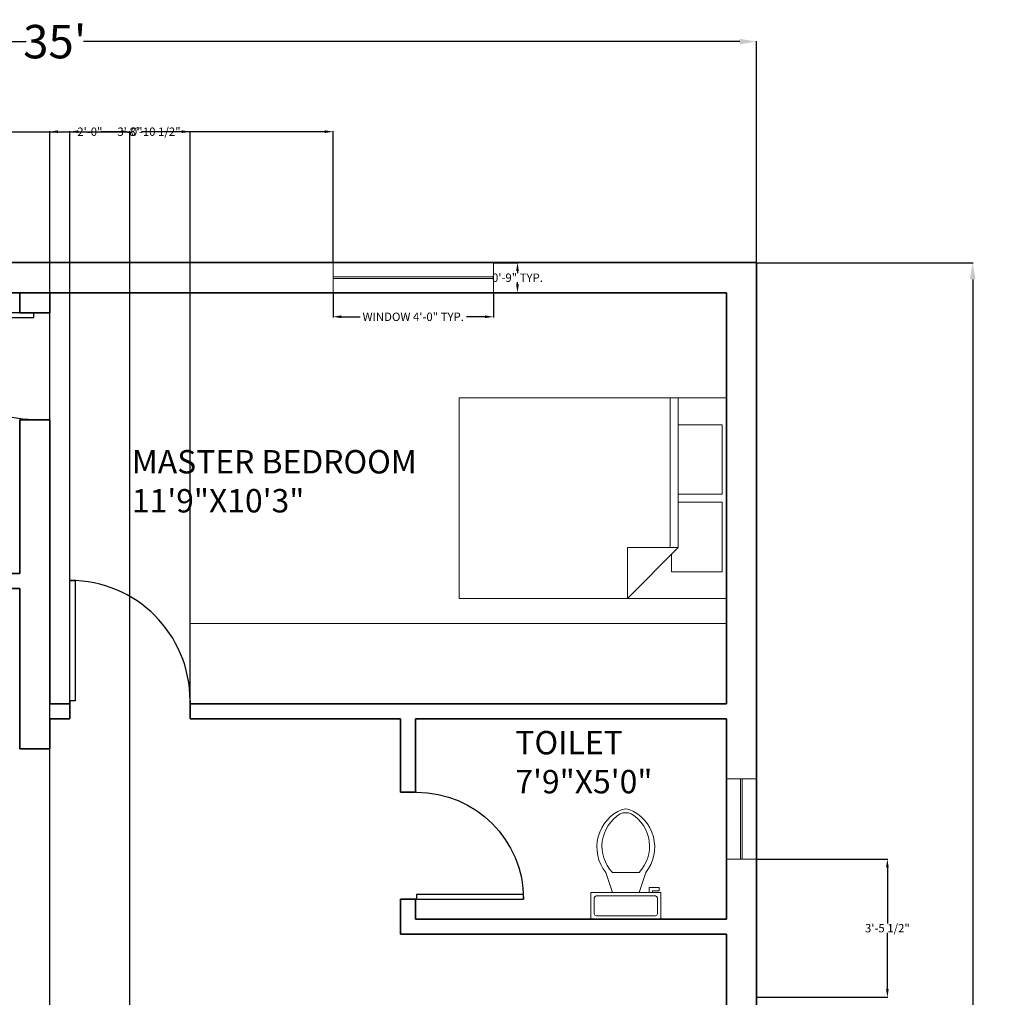
# Model space of a CAD drawing. Units: inches. Extents: x 481 to 2783, y 1975 to 3327.
# Tile 9 of 13: x 1574 to 1869, y 3034 to 3327. Entities that reach past the tile are written whole.
import ezdxf

# ---------------------------------------------------------------- set-up
doc = ezdxf.new("R2010")
doc.units = ezdxf.units.IN
doc.header["$MEASUREMENT"] = 0
for name, color, linetype, lineweight in [('A-ANNO-DIMS', 50, 'Continuous', 18), ('A-AREA-IDEN', 50, 'Continuous', 18), ('A-FLOR-CASE', 61, 'Continuous', 18), ('A-FLOR-FIXT', 61, 'Continuous', 18), ('A-FURN', 61, 'Continuous', 18), ('A-WALL', 40, 'Continuous', 35), ('DOORS', 10, 'Continuous', 25), ('WINDOWS', 220, 'Continuous', 20)]:
    doc.layers.add(name, color=color, linetype=linetype, lineweight=lineweight)
doc.styles.get("Standard").update_dxf_attribs({"font": 'arial.ttf'})
doc.dimstyles.get("Standard").update_dxf_attribs({"dimtxt": 2.5, "dimasz": 2.5, "dimexe": 0.18, "dimexo": 0.0625, "dimgap": 0.09, "dimtad": 0, "dimtih": 1, "dimtoh": 1, "dimzin": 0, "dimdsep": 46, "dimlunit": 3, "dimtxsty": 'Standard', "dimcen": 0.09, "dimadec": 0, "dimazin": 0, "dimtfac": 1, "dimtofl": 0, "dimtmove": 0, "dimatfit": 3, "dimfxl": 1, "dimtolj": 1, "dimtzin": 0, "dimarcsym": 0})

# ---------------------------------------------------------------- blocks, each defined once
blk = doc.blocks.new('*U2')
for p, q in [((0, 0), (0, -6)), ((40, 0), (40, -6))]:
    blk.add_line(p, q)
blk.add_lwpolyline([(0, 0), (0, 40), (1.75, 40), (1.75, 0)], close=True)
blk.add_arc((0, 0), 40, 0, 90)
blk = doc.blocks.new('Bed - Queen')
for p, q in [((0, -80.00003), (0, 0)), ((0, 0), (59.99999, 0)), ((59.99999, 0), (59.99999, -80.00003)), ((7.99999, -1.2), (28.79998, -1.2)), ((7.99999, -14.4), (7.99999, -1.2)), ((28.79998, -1.2), (28.79998, -14.4)), ((31.19999, -1.2), (51.99999, -1.2)), ((31.19999, -14.4), (31.19999, -1.2)), ((51.99999, -1.2), (51.99999, -16.4)), ((0, -14.4), (44.8, -14.4)), ((59.99999, -29.6), (44.8, -14.4)), ((44.8, -14.4), (44.8, -29.6)), ((44.8, -16.8), (0, -16.8)), ((51.99999, -16.4), (46.79936, -16.4)), ((44.8, -29.6), (59.99999, -29.6)), ((59.99999, -80.00003), (0, -80.00003))]:
    blk.add_line(p, q)
blk = doc.blocks.new('Toilet - top')
for p, q in [((9.5, -6), (9.5, -2)), ((-10, -8.5), (-8, -8.5)), ((-10, -9.5), (-10, -8.5)), ((-8, -8.5), (-8, -8)), ((-7, -8), (-7, -9.5)), ((-4, -8), (-6, -14)), ((4, -8), (6, -14)), ((-7, -9.5), (-10, -9.5)), ((4, -14), (-4, -14))]:
    blk.add_line(p, q)
blk.add_lwpolyline([(10.5, -8), (10.5, 0), (-10.5, 0), (-10.5, -8)], close=True)
for points in [[(-9.5, -2), (-9.5, -6)], [(8.5, -1), (-8.5, -1)], [(-8.5, -7), (8.5, -7)]]:
    blk.add_lwpolyline(points)
for centre, radius, start, end in [((-8.62, -1.88), 0.884, 81.8699, 188.1301), ((8.62, -1.88), 0.884, 351.8699, 98.1301), ((-8.62, -6.12), 0.884, 171.8699, 278.1301), ((8.62, -6.12), 0.884, 261.8699, 8.1301), ((3.52, -21.58), 12.17, 141.4691, 247.9714), ((4.2, -21.82), 11.33, 136.3677, 238.9468), ((-3.52, -21.58), 12.17, 292.0284, 38.5307), ((-4.2, -21.82), 11.33, 301.053, 43.6321), ((0, -27.88), 4, 245.7318, 294.2682), ((0, -29), 4, 254.8605, 285.1395)]:
    blk.add_arc(centre, radius, start, end)
blk = doc.blocks.new('*D23')
at = {"layer": 'A-ANNO-DIMS', "color": 0, "lineweight": -2, "transparency": 16777216}
for p, q in [((1794.5, 3254.32), (1859.35, 3254.32)), ((1859.17, 3249.32), (1859.17, 2959.52)), ((1859.17, 2659.32), (1859.17, 2949.13)), ((1794.5, 2654.32), (1859.35, 2654.32))]:
    blk.add_line(p, q, dxfattribs=at)
at = {"layer": 'A-ANNO-DIMS', "color": 0, "transparency": 16777216}
for points in [[(1858.33, 3249.32), (1860, 3249.32), (1859.17, 3254.32)], [(1858.33, 2659.32), (1860, 2659.32), (1859.17, 2654.32)]]:
    blk.add_solid(points, dxfattribs=at)
at = {"layer": 'Defpoints', "color": 0, "transparency": 16777216}
for p in [(1794.44, 3254.32), (1794.44, 2654.32), (1859.17, 2654.32)]:
    blk.add_point(p, dxfattribs=at)
at = {"layer": 'A-ANNO-DIMS', "color": 0, "transparency": 16777216, "insert": (1859.17, 2954.32), "char_height": 10, "attachment_point": 5}
blk.add_mtext("\\A1;50'", dxfattribs=at)
blk = doc.blocks.new('*D24')
at = {"layer": 'A-ANNO-DIMS', "color": 0, "lineweight": -2, "transparency": 16777216}
for p, q in [((1374.44, 3254.39), (1374.44, 3320.66)), ((1379.44, 3320.48), (1575.87, 3320.48)), ((1789.44, 3320.48), (1593.01, 3320.48)), ((1794.44, 3254.39), (1794.44, 3320.66))]:
    blk.add_line(p, q, dxfattribs=at)
at = {"layer": 'A-ANNO-DIMS', "color": 0, "transparency": 16777216}
for points in [[(1379.44, 3321.31), (1379.44, 3319.65), (1374.44, 3320.48)], [(1789.44, 3321.31), (1789.44, 3319.65), (1794.44, 3320.48)]]:
    blk.add_solid(points, dxfattribs=at)
at = {"layer": 'Defpoints', "color": 0, "transparency": 16777216}
for p in [(1794.44, 3320.48), (1374.44, 3254.32), (1794.44, 3254.32)]:
    blk.add_point(p, dxfattribs=at)
at = {"layer": 'A-ANNO-DIMS', "color": 0, "transparency": 16777216, "insert": (1584.44, 3320.48), "char_height": 10, "attachment_point": 5}
blk.add_mtext("\\A1;35'", dxfattribs=at)
blk = doc.blocks.new('WIN-PLAN-48IN')
for p, q in [((0, 4.75), (48, 4.75)), ((0, 4.25), (48, 4.25))]:
    blk.add_line(p, q)
blk.add_lwpolyline([(0, 0), (48, 0), (48, 9), (0, 9)], close=True)
blk = doc.blocks.new('WIN-PLAN-24IN')
for p, q in [((0, 4.75), (24, 4.75)), ((0, 4.25), (24, 4.25))]:
    blk.add_line(p, q)
blk.add_lwpolyline([(0, 0), (24, 0), (24, 9), (0, 9)], close=True)
blk = doc.blocks.new('*D28')
at = {"layer": 'A-ANNO-DIMS', "color": 0, "lineweight": -2, "transparency": 16777216}
for p, q in [((1667.73, 3245.26), (1667.73, 3237.94)), ((1715.73, 3245.26), (1715.73, 3237.94)), ((1670.23, 3238.12), (1675.82, 3238.12)), ((1713.23, 3238.12), (1707.63, 3238.12))]:
    blk.add_line(p, q, dxfattribs=at)
at = {"layer": 'A-ANNO-DIMS', "color": 0, "transparency": 16777216}
for points in [[(1670.23, 3238.54), (1670.23, 3237.71), (1667.73, 3238.12)], [(1713.23, 3238.54), (1713.23, 3237.71), (1715.73, 3238.12)]]:
    blk.add_solid(points, dxfattribs=at)
at = {"layer": 'Defpoints', "color": 0, "transparency": 16777216}
for p in [(1667.73, 3245.32), (1715.73, 3245.32), (1715.73, 3238.12)]:
    blk.add_point(p, dxfattribs=at)
at = {"layer": 'A-ANNO-DIMS', "color": 0, "transparency": 16777216, "insert": (1691.73, 3238.12), "char_height": 2.5, "attachment_point": 5}
blk.add_mtext('\\A1;WINDOW 4\'-0" TYP.', dxfattribs=at)
blk = doc.blocks.new('*D29')
at = {"layer": 'A-ANNO-DIMS', "color": 0, "lineweight": -2, "transparency": 16777216}
for p, q in [((1715.79, 3254.32), (1723.11, 3254.32)), ((1722.93, 3251.82), (1722.93, 3251.19)), ((1722.93, 3247.82), (1722.93, 3248.46)), ((1715.79, 3245.32), (1723.11, 3245.32))]:
    blk.add_line(p, q, dxfattribs=at)
at = {"layer": 'A-ANNO-DIMS', "color": 0, "transparency": 16777216}
for points in [[(1722.51, 3251.82), (1723.34, 3251.82), (1722.93, 3254.32)], [(1722.51, 3247.82), (1723.34, 3247.82), (1722.93, 3245.32)]]:
    blk.add_solid(points, dxfattribs=at)
at = {"layer": 'Defpoints', "color": 0, "transparency": 16777216}
for p in [(1715.73, 3254.32), (1722.93, 3254.32), (1715.73, 3245.32)]:
    blk.add_point(p, dxfattribs=at)
at = {"layer": 'A-ANNO-DIMS', "color": 0, "transparency": 16777216, "insert": (1722.93, 3249.82), "char_height": 2.5, "attachment_point": 5}
blk.add_mtext('\\A1;0\'-9" TYP.', dxfattribs=at)
blk = doc.blocks.new('*D85')
at = {"layer": 'A-ANNO-DIMS', "color": 0, "lineweight": -2, "transparency": 16777216}
for p, q in [((1561.13, 3254.39), (1561.13, 3293.7)), ((1563.63, 3293.52), (1607.13, 3293.52)), ((1665.23, 3293.52), (1621.72, 3293.52)), ((1667.73, 3254.39), (1667.73, 3293.7))]:
    blk.add_line(p, q, dxfattribs=at)
at = {"layer": 'A-ANNO-DIMS', "color": 0, "transparency": 16777216}
for points in [[(1563.63, 3293.94), (1563.63, 3293.11), (1561.13, 3293.52)], [(1665.23, 3293.94), (1665.23, 3293.11), (1667.73, 3293.52)]]:
    blk.add_solid(points, dxfattribs=at)
at = {"layer": 'Defpoints', "color": 0, "transparency": 16777216}
for p in [(1667.73, 3293.52), (1561.13, 3254.32), (1667.73, 3254.32)]:
    blk.add_point(p, dxfattribs=at)
at = {"layer": 'A-ANNO-DIMS', "color": 0, "transparency": 16777216, "insert": (1614.43, 3293.52), "char_height": 2.5, "attachment_point": 5}
blk.add_mtext('\\A1;8\'-10 1/2"', dxfattribs=at)
blk = doc.blocks.new('*D90')
at = {"layer": 'A-ANNO-DIMS', "color": 0, "lineweight": -2, "transparency": 16777216}
for p, q in [((1794.5, 3075.82), (1833.82, 3075.82)), ((1833.64, 3073.32), (1833.64, 3056.52)), ((1833.64, 3036.95), (1833.64, 3053.75)), ((1794.5, 3034.45), (1833.82, 3034.45))]:
    blk.add_line(p, q, dxfattribs=at)
at = {"layer": 'A-ANNO-DIMS', "color": 0, "transparency": 16777216}
for points in [[(1833.22, 3073.32), (1834.05, 3073.32), (1833.64, 3075.82)], [(1833.22, 3036.95), (1834.05, 3036.95), (1833.64, 3034.45)]]:
    blk.add_solid(points, dxfattribs=at)
at = {"layer": 'Defpoints', "color": 0, "transparency": 16777216}
for p in [(1794.44, 3075.82), (1833.64, 3075.82), (1794.44, 3034.45)]:
    blk.add_point(p, dxfattribs=at)
at = {"layer": 'A-ANNO-DIMS', "color": 0, "transparency": 16777216, "insert": (1833.64, 3055.14), "char_height": 2.5, "attachment_point": 5}
blk.add_mtext('\\A1;3\'-5 1/2"', dxfattribs=at)
blk = doc.blocks.new('*D99')
at = {"layer": 'A-ANNO-DIMS', "color": 0, "lineweight": -2, "transparency": 16777216}
for p, q in [((1588.94, 3122.39), (1588.94, 3293.7)), ((1591.44, 3293.52), (1603.53, 3293.52)), ((1622.44, 3293.52), (1610.35, 3293.52)), ((1624.94, 3122.39), (1624.94, 3293.7))]:
    blk.add_line(p, q, dxfattribs=at)
at = {"layer": 'A-ANNO-DIMS', "color": 0, "transparency": 16777216}
for points in [[(1591.44, 3293.94), (1591.44, 3293.11), (1588.94, 3293.52)], [(1622.44, 3293.94), (1622.44, 3293.11), (1624.94, 3293.52)]]:
    blk.add_solid(points, dxfattribs=at)
at = {"layer": 'Defpoints', "color": 0, "transparency": 16777216}
for p in [(1624.94, 3293.52), (1588.94, 3122.32), (1624.94, 3122.32)]:
    blk.add_point(p, dxfattribs=at)
at = {"layer": 'A-ANNO-DIMS', "color": 0, "transparency": 16777216, "insert": (1606.94, 3293.52), "char_height": 2.5, "attachment_point": 5}
blk.add_mtext('\\A1;3\'-0"', dxfattribs=at)
blk = doc.blocks.new('*D101')
at = {"layer": 'A-ANNO-DIMS', "color": 0, "lineweight": -2, "transparency": 16777216}
for p, q in [((1582.94, 2962.67), (1582.94, 3293.7)), ((1585.44, 3293.52), (1591.5, 3293.52)), ((1604.44, 3293.52), (1598.37, 3293.52)), ((1606.94, 2962.67), (1606.94, 3293.7))]:
    blk.add_line(p, q, dxfattribs=at)
at = {"layer": 'A-ANNO-DIMS', "color": 0, "transparency": 16777216}
for points in [[(1585.44, 3293.94), (1585.44, 3293.11), (1582.94, 3293.52)], [(1604.44, 3293.94), (1604.44, 3293.11), (1606.94, 3293.52)]]:
    blk.add_solid(points, dxfattribs=at)
at = {"layer": 'Defpoints', "color": 0, "transparency": 16777216}
for p in [(1606.94, 3293.52), (1582.94, 2962.61), (1606.94, 2962.61)]:
    blk.add_point(p, dxfattribs=at)
at = {"layer": 'A-ANNO-DIMS', "color": 0, "transparency": 16777216, "insert": (1594.94, 3293.52), "char_height": 2.5, "attachment_point": 5}
blk.add_mtext('\\A1;2\'-0"', dxfattribs=at)

msp = doc.modelspace()

# ---------------------------------------------------------------- linework, layer by layer
at = {"layer": 'A-FLOR-CASE'}
msp.add_line((1785.438, 3146.323), (1624.938, 3146.323), dxfattribs=at)
at = {"layer": 'A-WALL'}
for p, q in [((1573.938, 3245.323), (1519.938, 3245.323)), ((1573.938, 3245.323), (1573.938, 3239.323)), ((1573.938, 3245.323), (1582.938, 3245.323)), ((1785.438, 3245.323), (1582.938, 3245.323)), ((1582.938, 3245.323), (1582.938, 3239.323)), ((1785.438, 3122.323), (1785.438, 3245.323)), ((1573.938, 3239.323), (1582.938, 3239.323)), ((1573.938, 3207.323), (1582.938, 3207.323)), ((1573.938, 3207.323), (1573.938, 3161.323)), ((1582.938, 3207.323), (1582.938, 3122.323)), ((1573.938, 3161.323), (1519.938, 3161.323)), ((1573.938, 3156.823), (1519.938, 3156.823)), ((1573.938, 3156.823), (1573.938, 3108.823)), ((1588.938, 3122.323), (1582.938, 3122.323)), ((1588.938, 3122.323), (1588.938, 3117.823)), ((1785.438, 3122.323), (1624.938, 3122.323)), ((1624.938, 3122.323), (1624.938, 3117.823)), ((1588.938, 3117.823), (1582.938, 3117.823)), ((1582.938, 3117.823), (1582.938, 3108.823)), ((1687.938, 3117.823), (1624.938, 3117.823)), ((1687.938, 3095.823), (1687.938, 3117.823)), ((1785.438, 3117.823), (1692.438, 3117.823)), ((1692.438, 3095.823), (1692.438, 3117.823)), ((1785.438, 3057.823), (1785.438, 3117.823)), ((1582.938, 3113.323), (1582.938, 3108.823)), ((1582.938, 3108.823), (1573.938, 3108.823)), ((1687.938, 3095.823), (1692.438, 3095.823)), ((1687.938, 3053.323), (1687.938, 3063.823)), ((1687.938, 3063.823), (1692.438, 3063.823)), ((1692.438, 3057.823), (1692.438, 3063.823)), ((1785.438, 3057.823), (1692.438, 3057.823)), ((1785.438, 3053.323), (1687.938, 3053.323)), ((1785.438, 2873.323), (1785.438, 3053.323))]:
    msp.add_line(p, q, dxfattribs=at)
msp.add_lwpolyline([(1794.438, 2864.323), (1794.438, 3254.323), (1374.438, 3254.323), (1374.438, 2654.323), (1582.938, 2654.323)], dxfattribs=at)

# ---------------------------------------------------------------- block references
at = {"layer": 'A-FLOR-FIXT', "rotation": 180}
msp.add_blockref('Toilet - top', (1755.344, 3057.823), dxfattribs=at)
at = {"layer": 'A-FURN', "rotation": 270}
msp.add_blockref('Bed - Queen', (1785.438, 3213.823), dxfattribs=at)
at = {"layer": 'DOORS', "xscale": -0.8, "yscale": 0.8, "zscale": 0.8}
for p, rotation in [((1578.138, 3239.323), 90), ((1692.738, 3063.823), 270)]:
    msp.add_blockref('*U2', p, dxfattribs=dict(at, rotation=rotation))
at = {"layer": 'DOORS', "xscale": 0.9, "yscale": 0.9, "zscale": 0.9}
msp.add_blockref('*U2', (1588.938, 3123.223), dxfattribs=at)
at = {"layer": 'WINDOWS'}
msp.add_blockref('WIN-PLAN-48IN', (1667.726, 3245.323), dxfattribs=at)
at = {"layer": 'WINDOWS', "rotation": 270.0000000000015}
msp.add_blockref('WIN-PLAN-24IN', (1785.438, 3099.823), dxfattribs=at)

# ---------------------------------------------------------------- texts
at = {"layer": 'A-AREA-IDEN', "char_height": 7, "attachment_point": 1}
for s, width, insert in [('MASTER BEDROOM\\P11\'9"X10\'3"', 97.50928, (1607.517, 3198.234)), ('TOILET\\P7\'9"X5\'0"', 43.33543, (1722.291, 3114.169))]:
    msp.add_mtext_dynamic_manual_height_columns(s, width=width, gutter_width=1, heights=[0], dxfattribs=dict(at, insert=insert))

# ---------------------------------------------------------------- dimensions: what is measured, and where the dimension line sits
at = {"layer": 'A-ANNO-DIMS'}
for p1, p2, distance, picture, middle in [((1374.438, 3254.323), (1794.438, 3254.323), 66.156, '*D24', (1584.438, 3320.479)), ((1794.438, 3254.323), (1794.438, 2654.323), 64.73, '*D23', (1859.168, 2954.323))]:
    dim = msp.add_aligned_dim(p1=p1, p2=p2, distance=distance, dimstyle='Standard', override={"dimtxt": 10, "dimasz": 5, "dimclrd": 0, "dimclre": 0, "dimclrt": 0}, dxfattribs=at)
    dim.commit()
    dim.dimension.update_dxf_attribs({"geometry": picture, "text_midpoint": middle})
for base, p1, p2, picture, middle in [((1667.726, 3293.523), (1561.126, 3254.323), (1667.726, 3254.323), '*D85', (1614.426, 3293.523)), ((1606.938, 3293.523), (1582.938, 2962.607), (1606.938, 2962.607), '*D101', (1594.938, 3293.523)), ((1624.938, 3293.523), (1588.938, 3122.323), (1624.938, 3122.323), '*D99', (1606.938, 3293.523))]:
    dim = msp.add_linear_dim(base=base, p1=p1, p2=p2, dimstyle='Standard', override={"dimdec": 1, "dimlfac": 1, "dimrnd": 0, "dimzin": 1, "dimdsep": 46, "dimlunit": 4, "dimfrac": 2}, dxfattribs=at)
    dim.commit()
    dim.dimension.update_dxf_attribs({"geometry": picture, "text_midpoint": middle})
dim = msp.add_linear_dim(base=(1722.926, 3254.323), p1=(1715.726, 3245.323), p2=(1715.726, 3254.323), angle=90, text='<> TYP.', dimstyle='Standard', override={"dimdec": 1, "dimlfac": 1, "dimrnd": 0, "dimzin": 1, "dimdsep": 46, "dimlunit": 4, "dimfrac": 2}, dxfattribs=at)
dim.commit()
dim.dimension.update_dxf_attribs({"geometry": '*D29', "text_midpoint": (1722.926, 3249.823)})
dim = msp.add_linear_dim(base=(1715.726, 3238.123), p1=(1667.726, 3245.323), p2=(1715.726, 3245.323), text='WINDOW <> TYP.', dimstyle='Standard', override={"dimdec": 1, "dimlfac": 1, "dimrnd": 0, "dimzin": 1, "dimdsep": 46, "dimlunit": 4, "dimfrac": 2}, dxfattribs=at)
dim.commit()
dim.dimension.update_dxf_attribs({"geometry": '*D28', "text_midpoint": (1691.726, 3238.123)})
dim = msp.add_linear_dim(base=(1833.638, 3075.823), p1=(1794.438, 3034.448), p2=(1794.438, 3075.823), angle=90, dimstyle='Standard', override={"dimdec": 1, "dimlfac": 1, "dimrnd": 0, "dimzin": 1, "dimdsep": 46, "dimlunit": 4, "dimfrac": 2}, dxfattribs=at)
dim.commit()
dim.dimension.update_dxf_attribs({"geometry": '*D90', "text_midpoint": (1833.638, 3055.135)})

doc.saveas('drawing.dxf')
